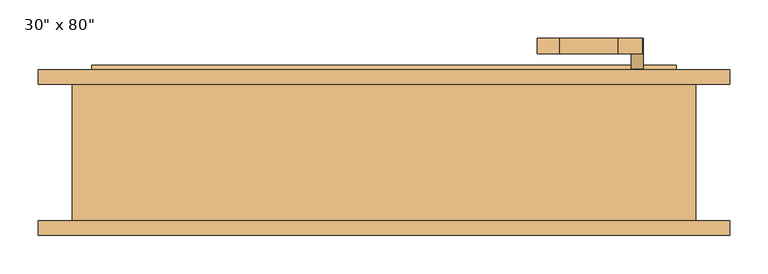
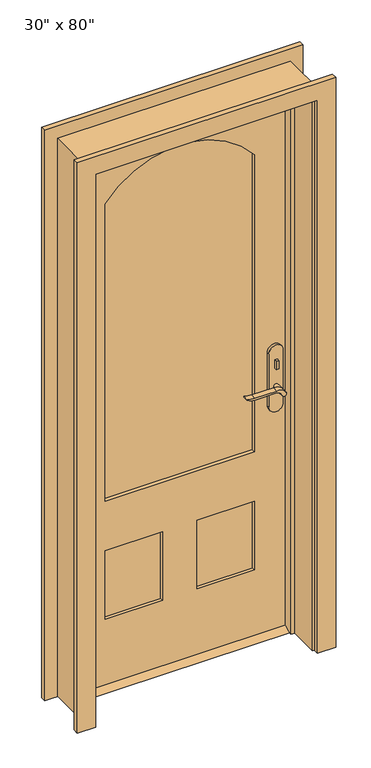
"""IFC4 building model written with IfcOpenShell, lengths in millimetres: door geometry."""

from ifc_helpers import new_model, si_unit, point, frame, frame_2d, origin, place, context, project, spatial, polyline, circle_curve, trimmed, segment, composite_curve, outline, extrude, faceted_brep, source, transform, mapped, element, save


def door_8a8e9806(model_context):
    return source(origin(), model_context, "Body", "SolidModel", [
        extrude(outline(polyline([(50.8, 12.7), (85.725, 12.7), (111.125, 0.0), (25.4, 0.0), (50.8, 12.7)])), frame((-381.0, 0.0, 0.0), z_axis=(1.0, 0.0, 0.0), x_axis=(0.0, 1.0, 0.0)), (0.0, 0.0, 1.0), 762.0),
        extrude(outline(polyline([(335.2, 30.8), (325.2, 30.8), (325.2, 40.8), (335.2, 40.8), (335.2, 30.8)])), frame((0.0, 0.0, 981.9), z_axis=(0.0, 0.0, 1.0), x_axis=(1.0, 0.0, 0.0)), (0.0, 0.0, 1.0), 30.0),
        extrude(outline(composite_curve([segment(trimmed(circle_curve(frame_2d((996.9, 330.2)), 8.0), [point((996.9, 322.2))], [point((996.9, 338.2))], False, "CARTESIAN"), True, "CONTINUOUS"), segment(trimmed(circle_curve(frame_2d((996.9, 330.2)), 8.0), [point((996.9, 338.2))], [point((996.9, 322.2))], False, "CARTESIAN"), True, "CONTINUOUS")], self_intersect=False)), frame((0.0, 95.725, 0.0), z_axis=(0.0, 1.0, 0.0), x_axis=(0.0, 0.0, 1.0)), (0.0, 0.0, 1.0), 10.0),
        extrude(outline(composite_curve([segment(trimmed(circle_curve(frame_2d((897.1555521, 306.5324871)), 37.2832219), [point((919.0523287, 336.7081363))], [point((934.4, 304.8325667))], False, "CARTESIAN"), True, "CONTINUOUS"), segment(polyline([(934.4, 304.8325667), (934.4, 228.5564091)]), True, "CONTINUOUS"), segment(trimmed(circle_curve(frame_2d((1017.6850638, 228.6227909)), 83.2850902), [point((934.4, 228.5564091))], [point((939.4, 200.2))], True, "CARTESIAN"), True, "CONTINUOUS"), segment(polyline([(939.4, 200.2), (936.6135558, 200.2)]), True, "CONTINUOUS"), segment(trimmed(circle_curve(frame_2d((986.6709207, 232.1396612)), 59.3791355), [point((936.6135558, 200.2))], [point((927.4, 228.5564091))], False, "CARTESIAN"), True, "CONTINUOUS"), segment(polyline([(927.4, 228.5564091), (927.4, 304.8138099)]), True, "CONTINUOUS"), segment(trimmed(circle_curve(frame_2d((909.2738613, 304.8138099)), 18.1261387), [point((927.4, 304.8138099))], [point((914.4, 322.2))], True, "CARTESIAN"), True, "CONTINUOUS"), segment(trimmed(circle_curve(frame_2d((914.4, 330.2)), 8.0), [point((914.4, 322.2))], [point((919.0523287, 336.7081363))], False, "CARTESIAN"), True, "CONTINUOUS")], self_intersect=False)), frame((0.0, -9.2, 0.0), z_axis=(0.0, 1.0, 0.0), x_axis=(0.0, 0.0, 1.0)), (0.0, 0.0, 1.0), 20.0),
        extrude(outline(composite_curve([segment(trimmed(circle_curve(frame_2d((914.4, 330.2)), 8.0), [point((914.3999903, 322.2))], [point((919.0523287, 336.7081363))], False, "CARTESIAN"), True, "CONTINUOUS"), segment(trimmed(circle_curve(frame_2d((897.1555521, 306.5324871)), 37.2832219), [point((919.0523287, 336.7081363))], [point((934.4, 304.8325667))], False, "CARTESIAN"), True, "CONTINUOUS"), segment(polyline([(934.4, 304.8325667), (934.4, 228.5564091)]), True, "CONTINUOUS"), segment(trimmed(circle_curve(frame_2d((1017.6850638, 228.6227909)), 83.2850902), [point((934.4, 228.5564091))], [point((939.4, 200.2))], True, "CARTESIAN"), True, "CONTINUOUS"), segment(polyline([(939.4, 200.2), (936.6135558, 200.2)]), True, "CONTINUOUS"), segment(trimmed(circle_curve(frame_2d((986.6709207, 232.1396612)), 59.3791355), [point((936.6135558, 200.2))], [point((927.4, 228.5564091))], False, "CARTESIAN"), True, "CONTINUOUS"), segment(polyline([(927.4, 228.5564091), (927.4, 304.8138122)]), True, "CONTINUOUS"), segment(trimmed(circle_curve(frame_2d((909.2738682, 304.8138122)), 18.1261318), [point((927.4, 304.8138122))], [point((914.3999903, 322.2))], True, "CARTESIAN"), True, "CONTINUOUS")], self_intersect=False)), frame((0.0, 125.725, 0.0), z_axis=(0.0, 1.0, 0.0), x_axis=(0.0, 0.0, 1.0)), (0.0, 0.0, 1.0), 20.0),
        extrude(outline(composite_curve([segment(trimmed(circle_curve(frame_2d((914.4, 330.2)), 8.0), [point((914.4, 322.2))], [point((914.4, 338.2))], False, "CARTESIAN"), True, "CONTINUOUS"), segment(trimmed(circle_curve(frame_2d((914.4, 330.2)), 8.0), [point((914.4, 338.2))], [point((914.4, 322.2))], False, "CARTESIAN"), True, "CONTINUOUS")], self_intersect=False)), frame((0.0, 10.8, 0.0), z_axis=(0.0, 1.0, 0.0), x_axis=(0.0, 0.0, 1.0)), (0.0, 0.0, 1.0), 30.0),
        extrude(outline(composite_curve([segment(trimmed(circle_curve(frame_2d((914.4, 330.2)), 8.0), [point((914.4, 322.2))], [point((914.4, 338.2))], False, "CARTESIAN"), True, "CONTINUOUS"), segment(trimmed(circle_curve(frame_2d((914.4, 330.2)), 8.0), [point((914.4, 338.2))], [point((914.4, 322.2))], False, "CARTESIAN"), True, "CONTINUOUS")], self_intersect=False)), frame((0.0, 95.725, 0.0), z_axis=(0.0, 1.0, 0.0), x_axis=(0.0, 0.0, 1.0)), (0.0, 0.0, 1.0), 30.0),
        extrude(outline(composite_curve([segment(polyline([(844.4, 355.2), (1039.4, 355.2)]), True, "CONTINUOUS"), segment(trimmed(circle_curve(frame_2d((1039.4, 330.2)), 25.0), [point((1039.4, 355.2))], [point((1039.4, 305.2))], False, "CARTESIAN"), True, "CONTINUOUS"), segment(polyline([(1039.4, 305.2), (844.4, 305.2)]), True, "CONTINUOUS"), segment(trimmed(circle_curve(frame_2d((844.4, 330.2)), 25.0), [point((844.4, 305.2))], [point((844.4, 355.2))], False, "CARTESIAN"), True, "CONTINUOUS")], self_intersect=False)), frame((0.0, 40.8, 0.0), z_axis=(0.0, 1.0, 0.0), x_axis=(0.0, 0.0, 1.0)), (0.0, 0.0, 1.0), 10.0),
        extrude(outline(composite_curve([segment(polyline([(844.4, 355.2), (1039.4, 355.2)]), True, "CONTINUOUS"), segment(trimmed(circle_curve(frame_2d((1039.4, 330.2)), 25.0), [point((1039.4, 355.2))], [point((1039.4, 305.2))], False, "CARTESIAN"), True, "CONTINUOUS"), segment(polyline([(1039.4, 305.2), (844.4, 305.2)]), True, "CONTINUOUS"), segment(trimmed(circle_curve(frame_2d((844.4, 330.2)), 25.0), [point((844.4, 305.2))], [point((844.4, 355.2))], False, "CARTESIAN"), True, "CONTINUOUS")], self_intersect=False)), frame((0.0, 85.725, 0.0), z_axis=(0.0, 1.0, 0.0), x_axis=(0.0, 0.0, 1.0)), (0.0, 0.0, 1.0), 10.0),
        extrude(outline(polyline([(2032.0, -381.0), (12.7, -381.0), (12.7, 381.0), (2032.0, 381.0), (2032.0, -381.0)]), holes=[composite_curve([segment(polyline([(688.975, -260.35), (1784.35, -260.35)]), True, "CONTINUOUS"), segment(trimmed(circle_curve(frame_2d((1580.99125, 0.0)), 330.35875), [point((1784.35, -260.35))], [point((1784.35, 260.35))], True, "CARTESIAN"), True, "CONTINUOUS"), segment(polyline([(1784.35, 260.35), (688.975, 260.35), (688.975, -260.35)]), True, "CONTINUOUS")], self_intersect=False), polyline([(508.0, -60.325), (254.0, -60.325), (254.0, -260.35), (508.0, -260.35), (508.0, -60.325)]), polyline([(508.0, 260.35), (254.0, 260.35), (254.0, 60.325), (508.0, 60.325), (508.0, 260.35)])]), frame((0.0, 50.8, 0.0), z_axis=(0.0, 1.0, 0.0), x_axis=(0.0, 0.0, 1.0)), (0.0, 0.0, 1.0), 34.925),
        faceted_brep([(406.4, 85.725, 0.0), (406.4, -92.075, 0.0), (381.0, -92.075, 0.0), (381.0, 15.875, 0.0), (368.3, 15.875, 0.0), (368.3, 50.8, 0.0), (381.0, 50.8, 0.0), (381.0, 85.725, 0.0), (406.4, 85.725, 2057.4), (406.4, -92.075, 2057.4), (-406.4, -92.075, 2057.4), (-406.4, -92.075, 0.0), (-381.0, -92.075, 0.0), (-381.0, -92.075, 2032.0), (381.0, -92.075, 2032.0), (381.0, 15.875, 2032.0), (-381.0, 15.875, 2032.0), (-381.0, 15.875, 0.0), (-368.3, 15.875, 0.0), (-368.3, 15.875, 2019.3), (368.3, 15.875, 2019.3), (368.3, 50.8, 2019.3), (-368.3, 50.8, 2019.3), (-368.3, 50.8, 0.0), (-381.0, 50.8, 0.0), (-381.0, 50.8, 2032.0), (381.0, 50.8, 2032.0), (381.0, 85.725, 2032.0), (-381.0, 85.725, 2032.0), (-381.0, 85.725, 0.0), (-406.4, 85.725, 0.0), (-406.4, 85.725, 2057.4)], [[[0, 1, 2, 3, 4, 5, 6, 7]], [[1, 0, 8, 9]], [[2, 1, 9, 10, 11, 12, 13, 14]], [[3, 2, 14, 15]], [[4, 3, 15, 16, 17, 18, 19, 20]], [[5, 4, 20, 21]], [[6, 5, 21, 22, 23, 24, 25, 26]], [[7, 6, 26, 27]], [[0, 7, 27, 28, 29, 30, 31, 8]], [[9, 8, 31, 10]], [[15, 14, 13, 16]], [[21, 20, 19, 22]], [[27, 26, 25, 28]], [[30, 29, 24, 23, 18, 17, 12, 11]], [[10, 31, 30, 11]], [[16, 13, 12, 17]], [[22, 19, 18, 23]], [[28, 25, 24, 29]]]),
        extrude(outline(polyline([(-60.325, 62.4416667), (-260.35, 62.4416667), (-260.35, 74.0833333), (-60.325, 74.0833333), (-60.325, 62.4416667)])), frame((0.0, 0.0, 254.0), z_axis=(0.0, 0.0, 1.0), x_axis=(1.0, 0.0, 0.0)), (0.0, 0.0, 1.0), 254.0),
        extrude(outline(polyline([(260.35, 62.4416667), (60.325, 62.4416667), (60.325, 74.0833333), (260.35, 74.0833333), (260.35, 62.4416667)])), frame((0.0, 0.0, 254.0), z_axis=(0.0, 0.0, 1.0), x_axis=(1.0, 0.0, 0.0)), (0.0, 0.0, 1.0), 254.0),
        extrude(outline(composite_curve([segment(polyline([(688.975, -260.35), (688.975, 260.35), (1784.35, 260.35)]), True, "CONTINUOUS"), segment(trimmed(circle_curve(frame_2d((1580.99125, 0.0)), 330.35875), [point((1784.35, 260.35))], [point((1784.35, -260.35))], False, "CARTESIAN"), True, "CONTINUOUS"), segment(polyline([(1784.35, -260.35), (688.975, -260.35)]), True, "CONTINUOUS")], self_intersect=False)), frame((0.0, 64.77, 0.0), z_axis=(0.0, 1.0, 0.0), x_axis=(0.0, 0.0, 1.0)), (0.0, 0.0, 1.0), 6.985),
        extrude(outline(polyline([(0.0, -450.85), (0.0, -387.35), (2038.35, -387.35), (2038.35, 387.35), (0.0, 387.35), (0.0, 450.85), (2101.85, 450.85), (2101.85, -450.85), (0.0, -450.85)])), frame((0.0, -111.125, 0.0), z_axis=(0.0, 1.0, 0.0), x_axis=(0.0, 0.0, 1.0)), (0.0, 0.0, 1.0), 19.05),
        extrude(outline(polyline([(0.0, -450.85), (0.0, -387.35), (2038.35, -387.35), (2038.35, 387.35), (0.0, 387.35), (0.0, 450.85), (2101.85, 450.85), (2101.85, -450.85), (0.0, -450.85)])), frame((0.0, 85.725, 0.0), z_axis=(0.0, 1.0, 0.0), x_axis=(0.0, 0.0, 1.0)), (0.0, 0.0, 1.0), 19.05),
    ])


if __name__ == "__main__":
    model = new_model("IFC4")
    model_context = context("Model", 3, world=origin())
    ifc_project = project(units=[si_unit("LENGTHUNIT", "METRE", prefix="MILLI")], contexts=[model_context])
    site = spatial("IfcSite", under=ifc_project)
    building = spatial("IfcBuilding", under=site)
    placement = place(None, origin())
    door_shape = door_8a8e9806(model_context)
    element("IfcDoor", 1, ObjectType="30\" x 80\"", at=placement, inside=building, context=model_context, shape_type="MappedRepresentation", body=[
        mapped(door_shape, transform((0.0, 0.0, 0.0), x_axis=(1.0, 0.0, 0.0), y_axis=(0.0, 1.0, 0.0), z_axis=(0.0, 0.0, 1.0))),
    ])
    save(model, "model.ifc")

# Revit data of these elements
# Type "30\" x 80\""
#   Type Mark = "9"
#   Assembly Code = "B2030100"
#   Analytic Construction = "French door, wood frame with single glass"
#   Threshold Offset [instance default] = 0' - 0 1/2"
#   Thickness = 0' - 1 3/8"
#   Thermal Resistance (R) = 1.0696 (h·ft²·°F)/BTU
#   Swing Angle [instance default] = 90.00°
#   Stiles = 0' - 4 3/4"
#   Rough Width = 2' - 8"
#   Rough Height = 6' - 9"
#   Radius = 1' - 1.00625"
#   Lock Rail = 0' - 7 1/8"
#   Height = 6' - 8"
#   Width = 2' - 6"
#   Heat Transfer Coefficient (U) = 0.9350 BTU/(h·ft²·°F)
#   Door Offset [instance default] = 0' - 0"
#   Bottom Rail = 0' - 9 1/2"
#   Threshold [instance default] = yes
#   Function = 1
#   Exterior Trim [instance default] = yes
#   Trim Material = Cherry
#   Threshold Material = Cherry
#   Panel Material = Cherry
#   Glazing = Glass
#   Frame Material = Cherry
#   Door Handle Material = Aluminum
#   Visual Light Transmittance = 0
#   Solar Heat Gain Coefficient = 0
#   Wall Closure = (empty or 0)
#   Construction Type = (empty or 0)
# Element 1 (IfcDoor, "30\" x 80\"")
#   Materials on its faces: "Cherry", "Aluminum", "Glass"
# Materials
#   "Cherry": class "Wood", colour RGB 226 177 128, transparency 0, Description = "Prunus Serotina", Cost = 0
#   "Glass": class "Glass", colour RGB 0 128 192, transparency 0.75, Description = "Soda Lime Glass", Cost = 0
#   "Aluminum": class "Metal", colour RGB 247 247 247, transparency 0, Description = "Aluminum 6061", Cost = 0
